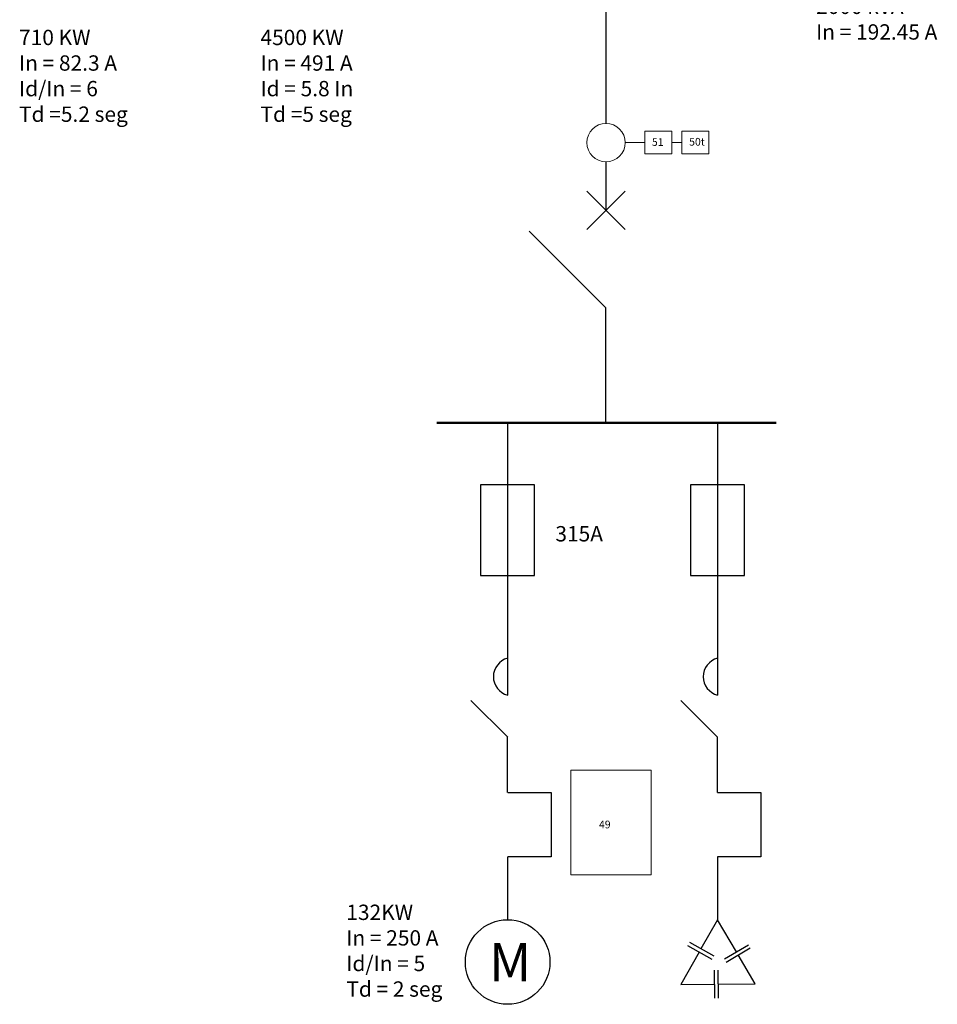
# Model space of a CAD drawing. Units: inches. Extents: x 77.1 to 95.7, y 45.4 to 81.6.
# Tile 1 of 3: x 77.1 to 89, y 45.4 to 58.2. Entities that reach past the tile are written whole.
import ezdxf

# ---------------------------------------------------------------- set-up
doc = ezdxf.new("R2010")
doc.units = ezdxf.units.IN
doc.header["$MEASUREMENT"] = 0
for name, color, linetype, lineweight in [('E-ANNO-TEXT', 7, 'Continuous', 18), ('E-POWR-BUSB', 7, 'Continuous', 50), ('E-POWR-CAPB', 3, 'Continuous', 25), ('E-POWR-CT', 4, 'Continuous', 18), ('E-POWR-EQPM', 3, 'Continuous', 30), ('E-POWR-FEED', 7, 'Continuous', 25), ('E-POWR-SWCH', 1, 'Continuous', 25), ('E-PROT-RELY', 2, 'Continuous', 18), ('E-PROT-TEXT', 7, 'Continuous', 13), ('E-PROT-WIRE', 5, 'Continuous', 13)]:
    doc.layers.add(name, color=color, linetype=linetype, lineweight=lineweight)
doc.styles.get("Standard").update_dxf_attribs({"font": 'arial.ttf'})

# ---------------------------------------------------------------- blocks, each defined once
blk = doc.blocks.new('CT-SINGLE')
blk.add_circle((0.25, 0.25), 0.25)
blk = doc.blocks.new('FUSE-LV')
for p, q in [((0.701, 1.182), (0, 1.182)), ((0, 1.182), (0, 0)), ((0.701, 0), (0.701, 1.182)), ((0, 0), (0.353, 0)), ((0.353, 0), (0.701, 0))]:
    blk.add_line(p, q)
blk = doc.blocks.new('SWITCH-LV-OPEN')
blk.add_line((0.481, 0), (0, 0.481))
blk.add_arc((0.542, 0.79), 0.248, 104.3094, 255.6906)
blk = doc.blocks.new('RELAY-FUNCTION')
for p, q in [((0, 0.148), (0, 0.295)), ((0, 0.295), (0.353, 0.295)), ((0.353, 0.295), (0.353, 0.148)), ((0, 0.148), (0, 0)), ((0.353, 0), (0.353, 0.148)), ((0, 0), (0.353, 0))]:
    blk.add_line(p, q)
blk = doc.blocks.new('OVERLOAD-ELEMENT')
for p, q in [((0, 0.838), (0.565, 0.838)), ((0.565, 0.838), (0.565, 0)), ((0.565, 0), (0, 0))]:
    blk.add_line(p, q)

msp = doc.modelspace()

# ---------------------------------------------------------------- linework, layer by layer
at = {"layer": 'E-POWR-BUSB'}
msp.add_line((82.519, 52.953), (86.943, 52.953), dxfattribs=at)
at = {"layer": 'E-POWR-CAPB'}
for p, q in [((86.109, 45.959), (85.792, 46.137)), ((86.132, 46.001), (85.816, 46.179)), ((86.267, 45.966), (86.58, 46.151)), ((86.292, 45.924), (86.605, 46.109)), ((86.134, 45.817), (86.138, 45.454)), ((86.182, 45.818), (86.186, 45.454))]:
    msp.add_line(p, q, dxfattribs=at)
for points in [[(86.424, 46.058), (86.178, 46.477), (85.962, 46.097)], [(85.938, 46.055), (85.699, 45.633), (86.136, 45.636)], [(86.184, 45.636), (86.669, 45.639), (86.448, 46.017)]]:
    msp.add_lwpolyline(points, dxfattribs=at)
at = {"layer": 'E-POWR-EQPM'}
msp.add_circle((83.443, 45.925), 0.551, dxfattribs=at)
at = {"layer": 'E-POWR-FEED'}
for p, q in [((84.724, 59.133), (84.724, 56.856)), ((84.724, 56.356), (84.724, 55.724)), ((84.724, 54.032), (84.724, 54.453)), ((84.724, 53.674), (84.724, 54.032)), ((84.724, 52.953), (84.724, 53.674)), ((83.443, 52.953), (83.443, 50.963)), ((86.179, 52.953), (86.179, 50.963)), ((83.443, 50.963), (83.443, 49.404)), ((86.179, 50.963), (86.179, 49.404)), ((83.443, 48.133), (83.443, 48.854)), ((86.179, 48.133), (86.179, 48.854)), ((83.443, 47.295), (83.443, 46.476)), ((86.179, 47.295), (86.179, 46.476))]:
    msp.add_line(p, q, dxfattribs=at)
at = {"layer": 'E-POWR-SWCH'}
for p, q in [((84.474, 55.474), (84.974, 55.974)), ((84.474, 55.974), (84.974, 55.474)), ((84.724, 54.453), (83.724, 55.453))]:
    msp.add_line(p, q, dxfattribs=at)
at = {"layer": 'E-PROT-RELY'}
msp.add_lwpolyline([(84.265, 48.427), (85.312, 48.427), (85.312, 47.06), (84.265, 47.06)], close=True, dxfattribs=at)
at = {"layer": 'E-PROT-WIRE'}
for p, q in [((84.974, 56.606), (85.231, 56.606)), ((85.583, 56.606), (85.712, 56.606))]:
    msp.add_line(p, q, dxfattribs=at)

# ---------------------------------------------------------------- block references
at = {"layer": 'E-POWR-CT'}
msp.add_blockref('CT-SINGLE', (84.475, 56.355), dxfattribs=at)
at = {"layer": 'E-POWR-SWCH'}
for name, p in [('FUSE-LV', (83.091, 50.963)), ('FUSE-LV', (85.826, 50.963)), ('SWITCH-LV-OPEN', (82.963, 48.854)), ('SWITCH-LV-OPEN', (85.698, 48.854)), ('OVERLOAD-ELEMENT', (83.444, 47.295)), ('OVERLOAD-ELEMENT', (86.179, 47.295))]:
    msp.add_blockref(name, p, dxfattribs=at)
at = {"layer": 'E-PROT-RELY'}
for p in [(85.231, 56.458), (85.712, 56.458)]:
    msp.add_blockref('RELAY-FUNCTION', p, dxfattribs=at)

# ---------------------------------------------------------------- texts
at = {"layer": 'E-ANNO-TEXT', "char_height": 0.2, "attachment_point": 1}
for s, width, insert in [('2000 kVA\\PIn = 192.45 A', 2.97281, (87.462, 58.481)), ('710 KW\\PIn = 82.3 A\\PId/In = 6\\PTd =5.2 seg', 2.97281, (77.077, 58.076)), ('4500 KW\\PIn = 491 A\\PId = 5.8 In\\PTd =5 seg', 2.97281, (80.223, 58.076)), ('315A', 0.93095, (84.065, 51.607)), ('132KW\\PIn = 250 A\\PId/In = 5\\PTd = 2 seg', 2.97281, (81.341, 46.673))]:
    msp.add_mtext_dynamic_manual_height_columns(s, width=width, gutter_width=1, heights=[0], dxfattribs=dict(at, insert=insert))
at = {"layer": 'E-POWR-EQPM', "insert": (83.199, 46.175), "char_height": 0.5, "attachment_point": 1}
msp.add_mtext_dynamic_manual_height_columns('M', width=0.27964, gutter_width=1, heights=[0], dxfattribs=at)
at = {"layer": 'E-PROT-TEXT', "char_height": 0.1, "attachment_point": 1}
for s, insert in [('51', (85.323, 56.663)), ('50t', (85.808, 56.666)), ('49', (84.633, 47.768))]:
    msp.add_mtext_dynamic_manual_height_columns(s, width=0.27964, gutter_width=1, heights=[0], dxfattribs=dict(at, insert=insert))

doc.saveas('drawing.dxf')
